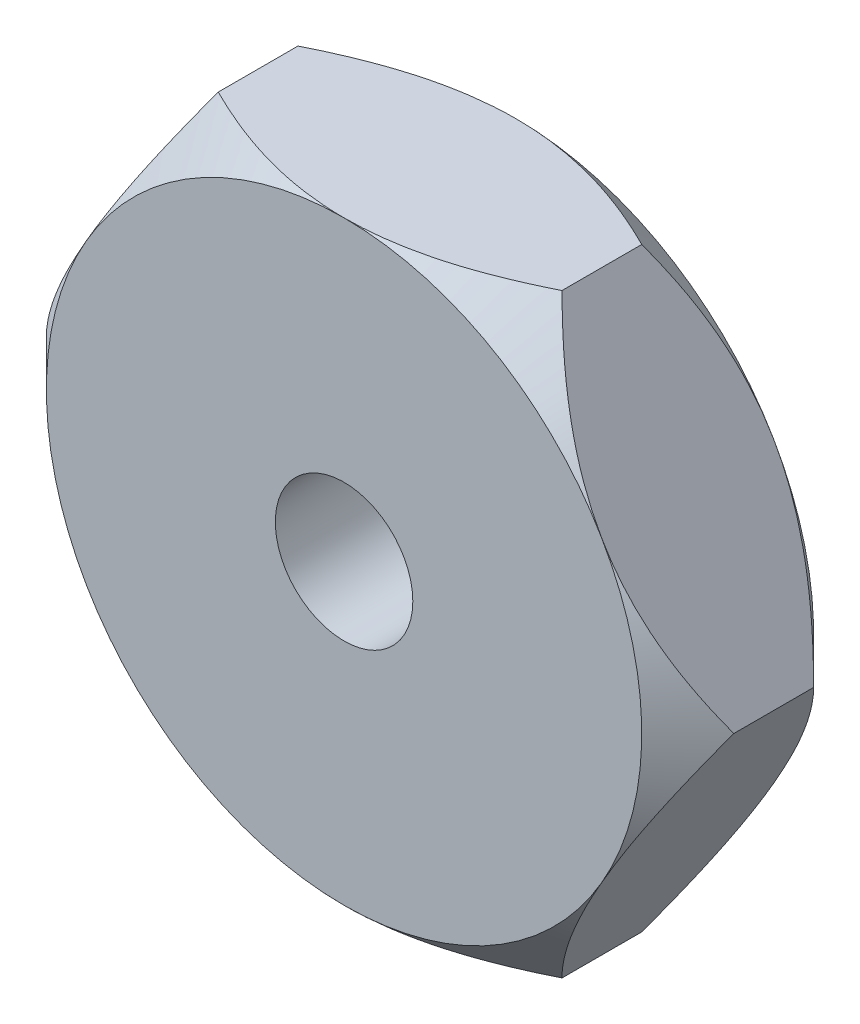
from build123d import *

# Parameters (mm, degrees)
HEX_BODY_DEPTH                        = 2.5
BORE_SKETCH_R                         = 2
BORE_4_DEPTH                          = 15.142135624
CORNER_CHAMFER_SKETCH_OUTSIDE_W       = 37.386
CORNER_CHAMFER_SKETCH_OUTSIDE_H       = 34.706
CORNER_CHAMFER_SKETCH_OUTSIDE_R       = 8.660254038
CORNER_CHAMFER_45DEG_DEPTH            = 5
CORNER_CHAMFER_45DEG_DRAFT            = -45
CORNER_CHAMFER_MIRROR_COPY_1_SKETCH_W = 37.386
CORNER_CHAMFER_MIRROR_COPY_1_SKETCH_H = 34.706
CORNER_CHAMFER_MIRROR_COPY_1_SKETCH_R = 8.660254038
CORNER_CHAMFER_MIRROR_COPY_1_DEPTH    = 5
CORNER_CHAMFER_MIRROR_COPY_1_DRAFT    = -45


with BuildPart() as part:
    # Hex Profile Sketch → Hex Body (new, symmetric)
    with BuildSketch(Plane.XY):
        Polygon((10, 0), (5, 8.660254038), (-5, 8.660254038), (-10, 0), (-5, -8.660254038), (5, -8.660254038), align=None)
    extrude(amount=HEX_BODY_DEPTH, both=True)

    # Bore Sketch → Bore Ø4 (cut, through all)
    with BuildSketch(Plane.XY.offset(2.5)):
        Circle(BORE_SKETCH_R)
    extrude(amount=-BORE_4_DEPTH, mode=Mode.SUBTRACT)


with BuildPart() as corner_chamfer_45deg_tool:
    # Corner Chamfer Sketch outside → Corner Chamfer 45deg (with draft: the straight prism first)
    with BuildSketch(Plane.XY.offset(2.5)):
        Rectangle(CORNER_CHAMFER_SKETCH_OUTSIDE_W, CORNER_CHAMFER_SKETCH_OUTSIDE_H)
        Circle(CORNER_CHAMFER_SKETCH_OUTSIDE_R, mode=Mode.SUBTRACT)
    extrude(amount=-CORNER_CHAMFER_45DEG_DEPTH)
    # Corner Chamfer 45deg: the draft: its side faces are tilted about the plane it starts from
    corner_chamfer_45deg_sides = [corner_chamfer_45deg_tool.faces().sort_by_distance(p)[0] for p in [
        (0, -17.353, 0),
        (18.693, 0, 0),
        (0, 17.353, 0),
        (-18.693, 0, 0),
        (-8.660254038, 0, 0),
    ]]
    draft(corner_chamfer_45deg_sides, Plane.XY.offset(2.5), CORNER_CHAMFER_45DEG_DRAFT)


with BuildPart() as part_1:
    add(part.part)

    # Corner Chamfer 45deg: cut by corner_chamfer_45deg_tool
    add(corner_chamfer_45deg_tool.part, mode=Mode.SUBTRACT)


with BuildPart() as corner_chamfer_mirror_copy_1_tool:
    # Corner Chamfer Mirror copy 1 sketch → Corner Chamfer Mirror copy 1 (with draft: the straight prism first)
    with BuildSketch(Plane(origin=(0, 0, -2.5), x_dir=(1, 0, 0), z_dir=(0, 0, -1))):
        Rectangle(CORNER_CHAMFER_MIRROR_COPY_1_SKETCH_W, CORNER_CHAMFER_MIRROR_COPY_1_SKETCH_H)
        Circle(CORNER_CHAMFER_MIRROR_COPY_1_SKETCH_R, mode=Mode.SUBTRACT)
    extrude(amount=-CORNER_CHAMFER_MIRROR_COPY_1_DEPTH)
    # Corner Chamfer Mirror copy 1: the draft: its side faces are tilted about the plane it starts from
    corner_chamfer_mirror_copy_1_sides = [corner_chamfer_mirror_copy_1_tool.faces().sort_by_distance(p)[0] for p in [
        (0, -17.353, 0),
        (18.693, 0, 0),
        (0, 17.353, 0),
        (-18.693, 0, 0),
        (-8.660254038, 0, 0),
    ]]
    draft(corner_chamfer_mirror_copy_1_sides, Plane(origin=(0, 0, -2.5), x_dir=(1, 0, 0), z_dir=(0, 0, -1)), CORNER_CHAMFER_MIRROR_COPY_1_DRAFT)


with BuildPart() as part_2:
    add(part_1.part)

    # Corner Chamfer Mirror copy 1: cut by corner_chamfer_mirror_copy_1_tool
    add(corner_chamfer_mirror_copy_1_tool.part, mode=Mode.SUBTRACT)


solid = part_2.part
